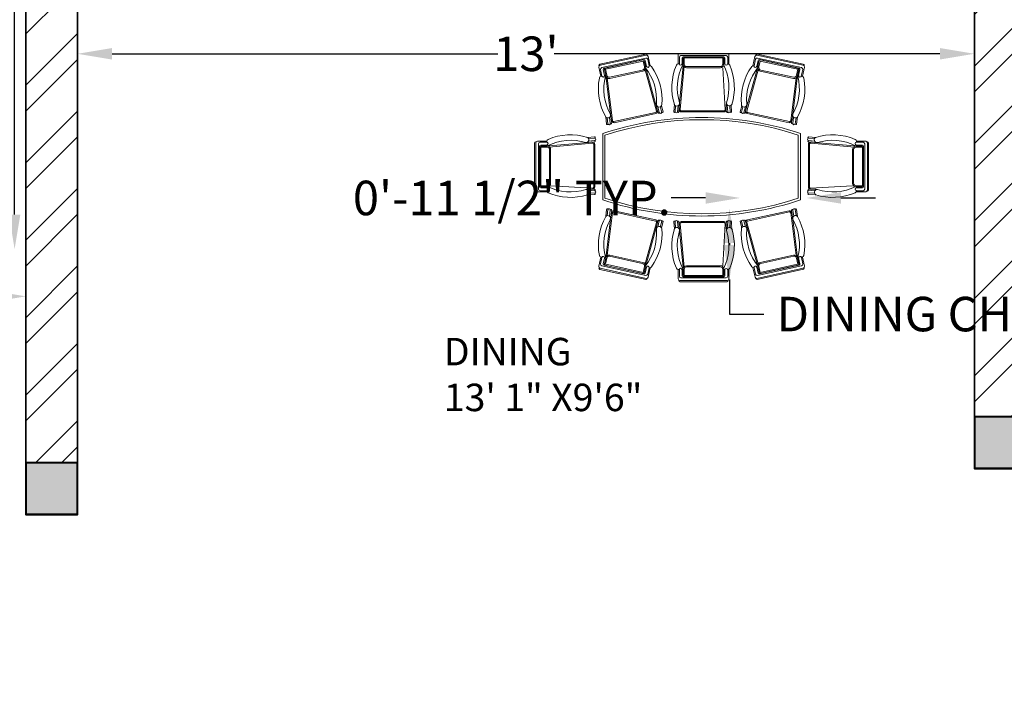
# Model space of a CAD drawing. Units: inches. Extents: x 3614 to 4242, y 2406 to 3033.
# Tile 7 of 10: x 3808 to 3980, y 2749 to 2864. Entities that reach past the tile are written whole.
import ezdxf

# ---------------------------------------------------------------- set-up
doc = ezdxf.new("R2010")
doc.units = ezdxf.units.IN
for name, color, linetype, lineweight in [('A-ANNO-DIMS', 2, 'Continuous', 18), ('A-AREA-IDEN', 7, 'Continuous', 25), ('A-COLS', 7, 'Continuous', 40), ('A-COLS-PATT', 252, 'Continuous', 18), ('A-FURN', 8, 'Continuous', 18), ('A-WALL', 7, 'Continuous', 35), ('A-WALL-PATT', 252, 'Continuous', 13)]:
    doc.layers.add(name, color=color, linetype=linetype, lineweight=lineweight)
doc.styles.get("Standard").update_dxf_attribs({"font": 'arial.ttf'})
doc.dimstyles.get("Standard").update_dxf_attribs({"dimtxt": 6, "dimasz": 6, "dimexe": 0.18, "dimexo": 0.0625, "dimgap": 0.09, "dimtad": 0, "dimtih": 1, "dimtoh": 1, "dimdec": 4, "dimzin": 0, "dimdsep": 46, "dimlunit": 4, "dimtxsty": 'Standard', "dimcen": 0.09, "dimse1": 1, "dimse2": 1, "dimadec": 0, "dimazin": 0, "dimtfac": 1, "dimtdec": 4, "dimtofl": 0, "dimtmove": 0, "dimatfit": 3, "dimfxl": 1, "dimtolj": 1, "dimtzin": 0, "dimarcsym": 0})

# ---------------------------------------------------------------- blocks, each defined once
blk = doc.blocks.new('*D14')
at = {"layer": 'A-ANNO-DIMS', "color": 0, "lineweight": -2, "transparency": 16777216}
for p, q in [((3824.34, 2858.42), (3891.44, 2858.42)), ((3968.34, 2858.42), (3901.24, 2858.42))]:
    blk.add_line(p, q, dxfattribs=at)
at = {"layer": 'A-ANNO-DIMS', "color": 0, "transparency": 16777216}
for points in [[(3824.34, 2859.42), (3824.34, 2857.42), (3818.34, 2858.42)], [(3968.34, 2859.42), (3968.34, 2857.42), (3974.34, 2858.42)]]:
    blk.add_solid(points, dxfattribs=at)
at = {"layer": 'Defpoints', "color": 0, "transparency": 16777216}
for p in [(3974.34, 2858.42), (3818.34, 2819.44), (3974.34, 2819.44)]:
    blk.add_point(p, dxfattribs=at)
at = {"layer": 'A-ANNO-DIMS', "color": 0, "transparency": 16777216, "insert": (3896.34, 2858.42), "char_height": 6, "attachment_point": 5}
blk.add_mtext("\\A1;13'", dxfattribs=at)
blk = doc.blocks.new('*D16')
at = {"layer": 'A-ANNO-DIMS', "color": 0, "lineweight": -2, "transparency": 16777216}
for p, q in [((3703.34, 2816.24), (3745.27, 2816.24)), ((3803.34, 2816.24), (3761.4, 2816.24))]:
    blk.add_line(p, q, dxfattribs=at)
at = {"layer": 'A-ANNO-DIMS', "color": 0, "transparency": 16777216}
for points in [[(3703.34, 2817.24), (3703.34, 2815.24), (3697.34, 2816.24)], [(3803.34, 2817.24), (3803.34, 2815.24), (3809.34, 2816.24)]]:
    blk.add_solid(points, dxfattribs=at)
at = {"layer": 'Defpoints', "color": 0, "transparency": 16777216}
for p in [(3809.34, 2816.24), (3697.34, 2813.05), (3809.34, 2813.05)]:
    blk.add_point(p, dxfattribs=at)
at = {"layer": 'A-ANNO-DIMS', "color": 0, "transparency": 16777216, "insert": (3753.34, 2816.24), "char_height": 6, "attachment_point": 5}
blk.add_mtext('\\A1;9\'-4"', dxfattribs=at)
blk = doc.blocks.new('COLUMN-9X9')
blk.add_lwpolyline([(9, 9), (0, 9), (0, 0), (9, 0)], close=True)
blk = doc.blocks.new('CHAIR-DINING')
for p, q in [((8.3, 12.29), (0.27, 10.54)), ((8.34, 12.11), (0.31, 10.36)), ((8.25, 11.6), (0.6, 9.93)), ((7.92, 11.33), (1.01, 9.82)), ((2.05, 10.02), (7.75, 11.27)), ((2.09, 9.83), (7.79, 11.08)), ((8.01, 10.07), (7.79, 11.08)), ((8.2, 10.12), (7.98, 11.12)), ((8.37, 10.16), (8.15, 11.19)), ((8.84, 10.26), (8.59, 11.38)), ((9.03, 10.26), (8.68, 11.89)), ((0.09, 10.01), (0.44, 8.43)), ((0.38, 9.59), (0.62, 8.47)), ((0.87, 9.6), (1.09, 8.57)), ((1.28, 8.57), (1.05, 9.61)), ((1.08, 8.6), (1.08, 8.6)), ((1.2, 9.84), (2.05, 10.02)), ((1.24, 9.65), (2.09, 9.83)), ((1.47, 8.61), (1.24, 9.65)), ((1.28, 8.55), (1.28, 8.57)), ((2.12, 1.84), (1.28, 8.57)), ((1.47, 8.61), (1.47, 8.58)), ((7.65, 9.5), (1.93, 8.25)), ((7.76, 9.33), (1.98, 8.07)), ((10.11, 2.37), (8.12, 9.58)), ((8.37, 10.15), (8.21, 10.12)), ((8.36, 9.41), (8.22, 9.89)), ((10.3, 2.43), (8.35, 9.46)), ((0.62, 8.47), (0.47, 8.44)), ((2.46, 0.71), (1.53, 8.15)), ((2.27, 0.69), (2.12, 1.84)), ((9.97, 2.14), (2.69, 0.55)), ((10.01, 1.95), (2.73, 0.36)), ((10.39, 2.07), (10.3, 2.4)), ((10.61, 2.12), (10.33, 3.14)), ((11.02, 2.2), (10.77, 3.12)), ((11.27, 2.24), (10.98, 3.3)), ((11.28, 2.23), (11.28, 2.23)), ((1.44, 0.11), (1.29, 1.36)), ((1.67, 0.16), (1.54, 1.21)), ((1.65, 0.13), (1.65, 0.13)), ((2.08, 0.25), (1.95, 1.29)), ((2.32, 0.31), (2.24, 0.93))]:
    blk.add_line(p, q)
for centre, radius, start, end in [((8.33, 12.1), 0.197, 12.3034, 102.3033), ((8.4, 11.83), 0.287, 12.3033, 102.303), ((0.37, 10.08), 0.287, 102.303, 192.3026), ((0.31, 10.35), 0.197, 102.3033, 212.9157), ((7.79, 11.08), 0.191, 12.3033, 102.3033), ((7.96, 11.14), 0.191, 12.3033, 102.303), ((8.31, 11.32), 0.287, 12.3033, 102.303), ((0.66, 9.65), 0.287, 102.303, 192.3026), ((0.84, 8.52), 0.242, 192.3034, 12.3032), ((1.05, 9.64), 0.191, 102.303, 192.3026), ((1.24, 9.65), 0.191, 102.3033, 192.3033), ((1.11, 8.42), 0.153, 71.7142, 102.3033), ((1.13, 8.47), 0.0956, 345.8699, 71.7142), ((1.85, 8.63), 0.382, 187.1284, 282.3033), ((7.55, 9.97), 0.478, 282.3033, 12.3033), ((7.64, 9.89), 0.573, 282.3033, 1.4878), ((8.23, 10.03), 0.0956, 102.3033, 218.7668), ((1.17, 4.36), 8.96, 354.9923, 38.7668), ((8.6, 10.22), 0.241, 194.1944, 8.7091), ((8.94, 9.89), 0.382, 35.4828, 104.8136), ((1.17, 4.36), 9.91, 354.9923, 35.4828), ((9.91, 6.26), 9.91, 169.1238, 209.6143), ((0.55, 8.06), 0.382, 102.3033, 169.1238), ((9.91, 6.26), 8.96, 165.8699, 209.6143), ((1.85, 8.63), 0.573, 187.1284, 282.3033), ((10.57, 3.55, -5.2), 0.477, 176.9365, 356.9364), ((1.66, 1.67), 0.477, 222.431, 27.6701), ((9.93, 2.32), 0.191, 282.3033, 15.4638), ((9.93, 2.32), 0.382, 282.3033, 15.4638), ((10.5, 2.1), 0.11, 193.7607, 13.7605), ((10.81, 2.17), 0.21, 192.3034, 12.3032), ((11.14, 2.23), 0.128, 193.5526, 13.5524), ((1.56, 0.14), 0.118, 192.3034, 12.3032), ((1.87, 0.21), 0.208, 192.3034, 12.3032), ((2.2, 0.28), 0.122, 193.4857, 13.4856), ((2.65, 0.74), 0.382, 187.1284, 282.3033), ((2.65, 0.74), 0.191, 187.1284, 282.3033)]:
    blk.add_arc(centre, radius, start, end)
blk = doc.blocks.new('*D45')
at = {"layer": 'A-ANNO-DIMS', "color": 0, "lineweight": -2, "transparency": 16777216}
for p, q in [((3931.73, 2825.5), (3931.73, 2825.16)), ((3931.73, 2819.16), (3931.73, 2813.16)), ((3931.73, 2813.16), (3937.73, 2813.16))]:
    blk.add_line(p, q, dxfattribs=at)
at = {"layer": 'A-ANNO-DIMS', "color": 0, "transparency": 16777216}
for points in [[(3932.73, 2825.5), (3930.73, 2825.5), (3931.73, 2831.5)], [(3932.73, 2825.16), (3930.73, 2825.16), (3931.73, 2819.16)]]:
    blk.add_solid(points, dxfattribs=at)
at = {"layer": 'Defpoints', "color": 0, "transparency": 16777216}
for p in [(3933.58, 2831.5), (3931.73, 2819.16), (3933.58, 2819.16)]:
    blk.add_point(p, dxfattribs=at)
at = {"layer": 'A-ANNO-DIMS', "color": 0, "transparency": 16777216, "insert": (3992.99, 2813.16), "char_height": 6, "attachment_point": 5}
blk.add_mtext('\\A1;DINING CHAIR 1\'-0 1/2" TYP.', dxfattribs=at)
blk = doc.blocks.new('*D46')
at = {"layer": 'A-ANNO-DIMS', "color": 0, "lineweight": -2, "transparency": 16777216}
for p, q in [((3927.58, 2833.35), (3921.58, 2833.35)), ((3951.13, 2833.36), (3957.13, 2833.36))]:
    blk.add_line(p, q, dxfattribs=at)
at = {"layer": 'A-ANNO-DIMS', "color": 0, "transparency": 16777216}
for points in [[(3927.58, 2834.35), (3927.58, 2832.35), (3933.58, 2833.35)], [(3951.13, 2834.36), (3951.13, 2832.36), (3945.13, 2833.35)]]:
    blk.add_solid(points, dxfattribs=at)
at = {"layer": 'Defpoints', "color": 0, "transparency": 16777216}
for p in [(3933.58, 2833.35), (3933.58, 2831.5), (3945.13, 2831.5)]:
    blk.add_point(p, dxfattribs=at)
at = {"layer": 'A-ANNO-DIMS', "color": 0, "transparency": 16777216, "insert": (3893.88, 2833.35), "char_height": 6, "attachment_point": 5}
blk.add_mtext('\\A1;0\'-11 1/2" TYP.', dxfattribs=at)
blk = doc.blocks.new('*D63')
at = {"layer": 'A-ANNO-DIMS', "color": 0, "lineweight": -2, "transparency": 16777216}
for p, q in [((3807.39, 2928.9), (3807.39, 2882.88)), ((3807.39, 2830.46), (3807.39, 2876.49))]:
    blk.add_line(p, q, dxfattribs=at)
at = {"layer": 'A-ANNO-DIMS', "color": 0, "transparency": 16777216}
for points in [[(3806.39, 2928.9), (3808.39, 2928.9), (3807.39, 2934.9)], [(3806.39, 2830.46), (3808.39, 2830.46), (3807.39, 2824.46)]]:
    blk.add_solid(points, dxfattribs=at)
at = {"layer": 'Defpoints', "color": 0, "transparency": 16777216}
for p in [(3790.82, 2934.9), (3807.39, 2934.9), (3790.82, 2824.46)]:
    blk.add_point(p, dxfattribs=at)
at = {"layer": 'A-ANNO-DIMS', "color": 0, "transparency": 16777216, "insert": (3807.39, 2879.68), "char_height": 6, "attachment_point": 5}
blk.add_mtext('\\A1;KITCHEN COUNTER 9\'-2 1/2"', dxfattribs=at)

msp = doc.modelspace()

# ---------------------------------------------------------------- hatches: boundary and pattern name
at = {"layer": 'A-COLS-PATT'}
h = msp.add_hatch(color=256, dxfattribs=at)
h.dxf.hatch_style = 1
h.paths.add_polyline_path([(3697.336, 2954.34049), (3688.336, 2954.34049), (3688.336, 2945.34049), (3697.336, 2945.34049)])
h.paths.add_polyline_path([(3818.336, 2954.34049), (3809.336, 2954.34049), (3809.336, 2945.34049), (3818.336, 2945.34049)])
h.paths.add_polyline_path([(3818.336, 2787.28572), (3809.336, 2787.28572), (3809.336, 2778.34049), (3818.336, 2778.34049)])
h.paths.add_polyline_path([(3697.336, 2742.34049), (3688.336, 2742.34049), (3688.336, 2733.34049), (3697.336, 2733.34049)])
h.paths.add_polyline_path([(3697.336, 2583.37355), (3688.336, 2583.37355), (3688.336, 2574.37355), (3697.336, 2574.37355)])
h.paths.add_polyline_path([(3899.336, 2583.34049), (3890.336, 2583.34049), (3890.336, 2574.34049), (3899.336, 2574.34049)])
h.paths.add_polyline_path([(3983.336, 2583.34049), (3974.336, 2583.34049), (3974.336, 2574.34049), (3983.336, 2574.34049)])
h.paths.add_polyline_path([(4153.336, 2583.34049), (4144.336, 2583.34049), (4144.336, 2574.34049), (4153.336, 2574.34049)])
h.paths.add_polyline_path([(4153.336, 2742.34049), (4144.336, 2742.34049), (4144.336, 2733.34049), (4153.336, 2733.34049)])
h.paths.add_polyline_path([(4153.336, 2795.34049), (4144.336, 2795.34049), (4144.336, 2786.34049), (4153.336, 2786.34049)])
h.paths.add_polyline_path([(3983.336, 2795.31105), (3974.336, 2795.31105), (3974.336, 2786.34049), (3983.336, 2786.34049)])
h.paths.add_polyline_path([(4153.336, 2954.34049), (4144.36882, 2954.34049), (4144.36882, 2945.34049), (4153.336, 2945.34049)])
h.paths.add_polyline_path([(3982.96188, 2954.34049), (3973.96188, 2954.34049), (3973.96188, 2945.34049), (3982.96188, 2945.34049)])
at = {"layer": 'A-WALL-PATT'}
h = msp.add_hatch(dxfattribs=at)
h.set_pattern_fill('ANSI32', color=256)
h.paths.add_polyline_path([(4041.01458, 2954.34049), (3982.96188, 2954.34049), (3982.96188, 2945.34049), (3983.336, 2945.34049), (4041.01458, 2945.34049)])
h.paths.add_polyline_path([(3973.96188, 2954.34049), (3960.11861, 2954.34049), (3960.11861, 2945.34049), (3973.96188, 2945.34049)])
h.paths.add_polyline_path([(3936.11861, 2954.34049), (3901.17016, 2954.34049), (3901.17016, 2945.34049), (3913.336, 2945.34049), (3913.336, 2896.34049, -0.050382044), (3919.336, 2895.73437), (3919.336, 2945.34049), (3936.11861, 2945.34049)])
h.paths.add_polyline_path([(3983.336, 2945.34049), (3982.96188, 2945.34049), (3974.336, 2945.34049), (3974.336, 2873.34049), (3974.336, 2795.31105), (3983.336, 2795.31105), (3983.336, 2867.34049)])
h.paths.add_polyline_path([(3974.336, 2872.34049), (3919.336, 2872.34049), (3858.336, 2872.34049), (3858.336, 2866.34049), (3919.336, 2866.34049), (3974.336, 2866.34049)])
h.paths.add_polyline_path([(3877.17016, 2954.34049), (3852.34021, 2954.34049), (3852.34021, 2945.34049), (3852.336, 2896.34049), (3858.336, 2896.34049), (3858.336, 2945.34049), (3877.17016, 2945.34049)])
h.paths.add_polyline_path([(3871.94212, 2902.34049), (3858.336, 2902.34049), (3858.336, 2896.34049), (3871.336, 2896.34049, -0.050382044)], flags=0)
h.paths.add_polyline_path([(3913.336, 2902.34049), (3901.336, 2902.34049), (3901.336, 2896.34049), (3913.336, 2896.34049)], flags=17)
h.paths.add_polyline_path([(3858.336, 2872.34049), (3852.336, 2872.34049), (3852.336, 2866.34049), (3858.336, 2866.34049)])
h.paths.add_polyline_path([(3809.336, 2954.34049), (3764.4617, 2954.34049), (3764.4617, 2945.34049), (3809.336, 2945.34049)])
h.paths.add_polyline_path([(3716.4617, 2954.34049), (3697.336, 2954.34049), (3697.336, 2945.34049), (3716.4617, 2945.34049)])
h.paths.add_polyline_path([(3697.336, 2945.34049), (3688.336, 2945.34049), (3688.336, 2894.73438), (3697.336, 2894.73438)])
h = msp.add_hatch(dxfattribs=at)
h.set_pattern_fill('ANSI32', color=256)
h.paths.add_polyline_path([(4153.336, 2945.34049), (4144.336, 2945.34049), (4144.336, 2902.95478), (4153.336, 2902.95478)])
h.paths.add_polyline_path([(4144.36882, 2954.34049), (4089.01458, 2954.34049), (4089.01458, 2945.34049), (4144.36882, 2945.34049)])
h.paths.add_polyline_path([(3818.336, 2945.34049), (3809.336, 2945.34049), (3809.336, 2787.28572), (3818.336, 2787.28572)])
h.paths.add_polyline_path([(3697.336, 2846.73438), (3688.336, 2846.73438), (3688.336, 2742.34049), (3697.336, 2742.34049)])
h.paths.add_polyline_path([(3854.336, 2742.34049), (3853.36389, 2742.34049), (3818.336, 2742.34049), (3809.336, 2742.34049), (3697.336, 2742.34049), (3697.336, 2733.34049), (3809.336, 2733.34049), (3854.336, 2733.34049)])
h.paths.add_polyline_path([(3697.336, 2733.34049), (3688.336, 2733.34049), (3688.336, 2690.05693), (3697.336, 2690.05693)])
h.paths.add_polyline_path([(3697.336, 2642.05693), (3688.336, 2642.05693), (3688.336, 2583.37355), (3697.336, 2583.37355)])
h.paths.add_polyline_path([(3726.39802, 2583.34049), (3697.336, 2583.34049), (3697.336, 2574.34049), (3726.39802, 2574.34049)])
h.paths.add_polyline_path([(3842.336, 2583.34049), (3818.336, 2583.34049), (3809.336, 2583.34049), (3774.39802, 2583.34049), (3774.39802, 2574.34049), (3809.336, 2574.34049), (3842.336, 2574.34049)])
h.paths.add_polyline_path([(3890.336, 2583.34049), (3878.336, 2583.34049), (3878.336, 2574.34049), (3890.336, 2574.34049)])
h = msp.add_hatch(dxfattribs=at)
h.set_pattern_fill('ANSI32', color=256)
h.paths.add_polyline_path([(3899.336, 2733.34049), (3899.336, 2742.34049), (3890.336, 2742.34049), (3890.336, 2583.34049), (3899.336, 2583.34049)])
h.paths.add_polyline_path([(3983.336, 2733.34049), (3995.336, 2733.34049), (3995.336, 2742.34049), (3983.336, 2742.34049), (3974.336, 2742.34049), (3974.336, 2583.34049), (3983.336, 2583.34049)])
h.paths.add_polyline_path([(3974.336, 2583.34049), (3899.336, 2583.34049), (3899.336, 2574.34049), (3974.336, 2574.34049)])
h.paths.add_polyline_path([(4045.73114, 2583.34049), (3983.336, 2583.34049), (3983.336, 2574.34049), (4045.73114, 2574.34049)])
h.paths.add_polyline_path([(4144.336, 2583.34049), (4093.73114, 2583.34049), (4093.73114, 2574.34049), (4144.336, 2574.34049)])
h.paths.add_polyline_path([(4153.336, 2639.00845), (4144.336, 2639.00845), (4144.336, 2583.34049), (4153.336, 2583.34049)])
h.paths.add_polyline_path([(4153.336, 2733.34049), (4144.336, 2733.34049), (4144.336, 2687.00845), (4153.336, 2687.00845)])
h.paths.add_polyline_path([(4144.336, 2742.34049), (4096.76112, 2742.34049, -0.076320834), (4098.14294, 2733.34049), (4144.336, 2733.34049)])
h.paths.add_polyline_path([(4068.14294, 2742.34049), (4056.14294, 2742.34049), (4031.336, 2742.34049, -0.063254224), (4030.19285, 2733.34049), (4068.14294, 2733.34049)])
h.paths.add_polyline_path([(4144.336, 2795.34049), (4042.336, 2795.34049), (4042.336, 2786.34049), (4144.336, 2786.34049)])
h.paths.add_polyline_path([(4153.336, 2854.95478), (4144.336, 2854.95478), (4144.336, 2795.34049), (4153.336, 2795.34049)])

# ---------------------------------------------------------------- linework, layer by layer
at = {"layer": 'A-FURN'}
for p, q in [((3922.82983, 2858.29837), (3922.82981, 2856.67394)), ((3923.02093, 2857.8206), (3923.02092, 2856.67394)), ((3931.14309, 2858.10721), (3923.3076, 2858.10726)), ((3923.49871, 2857.72504), (3923.49869, 2856.67393)), ((3923.68233, 2856.63157), (3923.68233, 2857.69683)), ((3930.76087, 2857.9161), (3923.68982, 2857.91615)), ((3923.87343, 2857.88793), (3930.58343, 2857.88793)), ((3923.87343, 2856.63157), (3923.87343, 2857.69683)), ((3923.87343, 2857.69683), (3930.58343, 2857.69683)), ((3930.58343, 2856.66104), (3930.58343, 2857.69683)), ((3930.77454, 2856.67065), (3930.77454, 2857.69683)), ((3930.95198, 2856.67389), (3930.95198, 2857.72499)), ((3931.42975, 2856.67389), (3931.42975, 2857.82054)), ((3931.62086, 2856.63232), (3931.62086, 2858.29832)), ((3923.01445, 2856.67441), (3922.86495, 2856.67441)), ((3923.07454, 2849.87451), (3923.65867, 2856.32445)), ((3923.16044, 2848.70423), (3923.85057, 2856.32445)), ((3923.49867, 2856.70429), (3923.49873, 2856.70491)), ((3923.68519, 2856.6172), (3923.68642, 2856.63078)), ((3930.10566, 2856.18327), (3924.25618, 2856.18327)), ((3930.17748, 2855.99216), (3924.25618, 2855.99216)), ((3930.99473, 2848.69753), (3930.59251, 2855.98182)), ((3930.9483, 2856.67065), (3930.78946, 2856.67065)), ((3930.94127, 2856.64313), (3930.93959, 2856.67171)), ((3931.43017, 2856.6484), (3931.429, 2856.67171)), ((3922.03956, 2848.33797), (3922.15359, 2849.59779)), ((3922.24897, 2848.30477), (3922.24904, 2848.30589)), ((3922.27521, 2848.33797), (3922.36724, 2849.38276)), ((3922.69211, 2848.33797), (3922.79272, 2849.38159)), ((3922.93698, 2848.34511), (3922.99185, 2848.96492)), ((3922.97011, 2848.72146), (3923.07454, 2849.87451)), ((3930.80391, 2848.49588), (3923.35077, 2848.49588)), ((3930.80391, 2848.30477), (3923.35077, 2848.30477)), ((3931.18555, 2848.70806), (3931.13769, 2849.57484)), ((3931.2038, 2848.34033), (3931.18226, 2848.68338)), ((3931.429, 2848.33797), (3931.35985, 2849.51543)), ((3931.84591, 2848.33797), (3931.79587, 2849.33815)), ((3932.09871, 2848.32111), (3932.03174, 2849.44774)), ((3932.09968, 2848.30477), (3932.09961, 2848.30589)), ((3898.32537, 2843.21638), (3899.9498, 2843.2164)), ((3899.94933, 2843.03177), (3899.94933, 2843.18126)), ((3908.28577, 2844.00665), (3907.02595, 2843.89262)), ((3908.28577, 2843.77101), (3907.24099, 2843.67897)), ((3908.28577, 2843.3541), (3907.24215, 2843.25349)), ((3908.31897, 2843.79724), (3908.31786, 2843.79717)), ((3909.69472, 2844.54018), (3909.69472, 2833.01769)), ((3910.07694, 2844.2642), (3910.07694, 2833.29345)), ((3943.71216, 2844.29393), (3943.71216, 2833.29033)), ((3944.09438, 2844.57043), (3944.09438, 2833.01451)), ((3945.46538, 2843.79724), (3945.4665, 2843.79717)), ((3945.49859, 2844.00665), (3946.7584, 2843.89262)), ((3945.49859, 2843.77101), (3946.54337, 2843.67897)), ((3945.49859, 2843.3541), (3946.54221, 2843.25349)), ((3955.45898, 2843.21638), (3953.83455, 2843.2164)), ((3953.83502, 2843.03177), (3953.83502, 2843.18126)), ((3897.84765, 2834.71201), (3897.8476, 2842.92972)), ((3898.03876, 2834.71202), (3898.03871, 2842.92972)), ((3898.51654, 2834.90312), (3898.51649, 2842.73861)), ((3898.70764, 2835.28534), (3898.7076, 2842.3564)), ((3898.73581, 2842.17278), (3898.73581, 2835.46278)), ((3898.80315, 2843.02528), (3899.9498, 2843.02529)), ((3898.8987, 2842.54751), (3899.94981, 2842.54752)), ((3899.99218, 2842.36389), (3898.92692, 2842.36389)), ((3898.92692, 2842.17278), (3898.92692, 2835.46278)), ((3899.99218, 2842.17278), (3898.92692, 2842.17278)), ((3899.91945, 2842.54754), (3899.91883, 2842.54748)), ((3900.00655, 2842.36103), (3899.99296, 2842.3598)), ((3907.90228, 2843.0761), (3900.29929, 2842.38754)), ((3907.91952, 2842.88577), (3900.29929, 2842.19565)), ((3900.44048, 2835.94056), (3900.44048, 2841.79004)), ((3900.63158, 2835.86873), (3900.63158, 2841.79004)), ((3908.27863, 2843.10923), (3907.65883, 2843.05436)), ((3908.12786, 2835.2423), (3908.12786, 2842.69544)), ((3908.31897, 2835.2423), (3908.31897, 2842.69544)), ((3945.46538, 2835.2423), (3945.46538, 2842.69544)), ((3945.50572, 2843.10923), (3946.12553, 2843.05436)), ((3945.65649, 2835.2423), (3945.65649, 2842.69544)), ((3945.86484, 2842.88577), (3953.48507, 2842.19565)), ((3945.88208, 2843.0761), (3953.48507, 2842.38754)), ((3953.15277, 2835.86873), (3953.15277, 2841.79004)), ((3953.34388, 2835.94056), (3953.34388, 2841.79004)), ((3953.77781, 2842.36103), (3953.79139, 2842.3598)), ((3953.79218, 2842.36389), (3954.85744, 2842.36389)), ((3953.79218, 2842.17278), (3954.85744, 2842.17278)), ((3954.98121, 2843.02528), (3953.83455, 2843.02529)), ((3954.88565, 2842.54751), (3953.83455, 2842.54752)), ((3953.86491, 2842.54754), (3953.86553, 2842.54748)), ((3954.85744, 2842.17278), (3954.85744, 2835.46278)), ((3955.04855, 2842.17278), (3955.04855, 2835.46278)), ((3955.07671, 2835.28534), (3955.07676, 2842.3564)), ((3955.26782, 2834.90312), (3955.26787, 2842.73861)), ((3955.74559, 2834.71202), (3955.74564, 2842.92972)), ((3955.9367, 2834.71201), (3955.93675, 2842.92972)), ((3899.94986, 2834.61646), (3898.8032, 2834.61646)), ((3899.94986, 2835.09424), (3898.89875, 2835.09424)), ((3899.9627, 2835.46278), (3898.92692, 2835.46278)), ((3899.95309, 2835.27168), (3898.92692, 2835.27168)), ((3899.98062, 2835.10494), (3899.95203, 2835.10662)), ((3899.97534, 2834.61605), (3899.95203, 2834.61721)), ((3899.95309, 2835.09791), (3899.95309, 2835.25676)), ((3907.92622, 2835.05148), (3900.64192, 2835.4537)), ((3907.91568, 2834.86066), (3907.0489, 2834.90852)), ((3908.28577, 2834.61721), (3907.10832, 2834.68636)), ((3908.28341, 2834.84241), (3907.94036, 2834.86396)), ((3945.49859, 2834.61721), (3946.67604, 2834.68636)), ((3945.50095, 2834.84241), (3945.84399, 2834.86396)), ((3945.85814, 2835.05148), (3953.14243, 2835.4537)), ((3945.86868, 2834.86066), (3946.73546, 2834.90852)), ((3953.80374, 2835.10494), (3953.83233, 2835.10662)), ((3953.80902, 2834.61605), (3953.83233, 2834.61721)), ((3953.82165, 2835.46278), (3954.85744, 2835.46278)), ((3953.83127, 2835.27168), (3954.85744, 2835.27168)), ((3953.83127, 2835.09791), (3953.83127, 2835.25676)), ((3953.8345, 2835.09424), (3954.8856, 2835.09424)), ((3953.8345, 2834.61646), (3954.98116, 2834.61646)), ((3899.99142, 2834.42535), (3898.32543, 2834.42535)), ((3908.30263, 2833.94751), (3907.17601, 2834.01447)), ((3908.28577, 2834.20031), (3907.28559, 2834.25034)), ((3908.31897, 2833.94654), (3908.31786, 2833.9466)), ((3945.46538, 2833.94654), (3945.4665, 2833.9466)), ((3945.48172, 2833.94751), (3946.60835, 2834.01447)), ((3945.49859, 2834.20031), (3946.49877, 2834.25034)), ((3953.79293, 2834.42535), (3955.45893, 2834.42535)), ((3922.03956, 2829.21982), (3922.15359, 2827.96001)), ((3922.24897, 2829.25302), (3922.24904, 2829.25191)), ((3922.27521, 2829.21982), (3922.36724, 2828.17504)), ((3922.69211, 2829.21982), (3922.79272, 2828.1762)), ((3922.93698, 2829.21269), (3922.99185, 2828.59288)), ((3922.97011, 2828.83633), (3923.07454, 2827.68329)), ((3923.16044, 2828.85357), (3923.85057, 2821.23334)), ((3930.80391, 2829.25302), (3923.35077, 2829.25302)), ((3930.80391, 2829.06192), (3923.35077, 2829.06192)), ((3930.99473, 2828.86027), (3930.59251, 2821.57598)), ((3931.18555, 2828.84973), (3931.13769, 2827.98295)), ((3931.2038, 2829.21746), (3931.18226, 2828.87442)), ((3931.429, 2829.21982), (3931.35985, 2828.04237)), ((3931.84591, 2829.21982), (3931.79587, 2828.21964)), ((3932.09871, 2829.23668), (3932.03174, 2828.11006)), ((3932.09968, 2829.25302), (3932.09961, 2829.25191)), ((3923.07454, 2827.68329), (3923.65867, 2821.23334)), ((3922.82983, 2819.25942), (3922.82981, 2820.88386)), ((3923.01445, 2820.88339), (3922.86495, 2820.88339)), ((3923.02093, 2819.7372), (3923.02092, 2820.88386)), ((3923.49867, 2820.8535), (3923.49873, 2820.85288)), ((3923.49871, 2819.83276), (3923.49869, 2820.88386)), ((3923.68233, 2820.92623), (3923.68233, 2819.86097)), ((3923.68519, 2820.9406), (3923.68642, 2820.92702)), ((3923.87343, 2820.92623), (3923.87343, 2819.86097)), ((3930.17748, 2821.56564), (3924.25618, 2821.56564)), ((3930.10566, 2821.37453), (3924.25618, 2821.37453)), ((3930.58343, 2820.89676), (3930.58343, 2819.86097)), ((3930.77454, 2820.88714), (3930.77454, 2819.86097)), ((3930.9483, 2820.88714), (3930.78946, 2820.88714)), ((3930.94127, 2820.91467), (3930.93959, 2820.88608)), ((3930.95198, 2820.88391), (3930.95198, 2819.8328)), ((3931.43017, 2820.90939), (3931.429, 2820.88608)), ((3931.42975, 2820.88391), (3931.42975, 2819.73725)), ((3931.62086, 2820.92548), (3931.62086, 2819.25948)), ((3931.14309, 2819.45059), (3923.3076, 2819.45054)), ((3930.76087, 2819.6417), (3923.68982, 2819.64165)), ((3923.87343, 2819.86097), (3930.58343, 2819.86097)), ((3923.87343, 2819.66986), (3930.58343, 2819.66986)), ((3931.3342, 2818.97282), (3923.1165, 2818.97276)), ((3931.3342, 2818.78171), (3923.1165, 2818.78166))]:
    msp.add_line(p, q, dxfattribs=at)
for centre, radius, start, end in [((3923.3076, 2857.82059), 0.28666, 89.9996381, 179.999275), ((3923.68982, 2857.72504), 0.19111, 89.9996381, 179.999275), ((3923.87343, 2857.69683), 0.19111, 90, 180), ((3930.58343, 2857.69683), 0.19111, 0, 90), ((3930.76087, 2857.72499), 0.19111, 0, 89.9996381), ((3931.14309, 2857.82054), 0.28666, 0, 89.9996381), ((3931.6278, 2852.54013), 9.91456, 156.8204824, 197.3110234), ((3922.86495, 2856.29219), 0.38222, 90, 156.8204824), ((3931.6278, 2852.54013), 8.95902, 153.5665946, 197.3110234), ((3923.24766, 2856.68072), 0.24162, 180.000076, 359.999924), ((3923.49057, 2856.52128), 0.15313, 59.410873, 90), ((3923.51987, 2856.57084), 0.09555, 333.5665946, 59.410873), ((3924.25618, 2856.56549), 0.57333, 174.8251214, 270), ((3931.6278, 2852.54013), 8.95902, 152.2307223, 152.4302915), ((3924.25618, 2856.56549), 0.38222, 174.8251214, 270), ((3930.10566, 2856.66104), 0.47777, 270, 0), ((3930.17748, 2856.56549), 0.57333, 270, 351.0504472), ((3930.78946, 2856.5751), 0.09555, 90, 206.4634741), ((3922.68363, 2852.54013), 8.95902, 342.6889766, 26.4634741), ((3931.1819, 2856.68072), 0.23333, 180.000076, 359.999924), ((3931.44649, 2856.29219), 0.38222, 23.1795176, 90), ((3922.68363, 2852.54013), 9.91456, 342.6889766, 23.1795176), ((3922.15697, 2848.33728), 0.1178, 180.000076, 359.999924), ((3922.58115, 2849.80894), 0.47686, 195.3669467, 15.3667947), ((3922.48298, 2848.33728), 0.20821, 180.000076, 359.999924), ((3922.81275, 2848.33979), 0.12159, 181.1824337, 1.1822816), ((3923.35077, 2848.68699), 0.38222, 174.8251214, 270), ((3923.35077, 2848.68699), 0.19111, 174.8251214, 270), ((3930.80391, 2848.68699), 0.38222, 270, 3.1605363), ((3930.80391, 2848.68699), 0.19111, 270, 3.1605363), ((3931.31411, 2848.34232), 0.10978, 181.4573887, 1.4572366), ((3931.7224, 2849.82282), 0.48828, 173.9478508, 343.3079431), ((3931.6342, 2848.34511), 0.21034, 180.000076, 359.999924), ((3931.96801, 2848.33673), 0.12807, 181.2492726, 1.2491205), ((3926.93992, 2792.95024), 54.39594, 71.6172783, 108.4834683), ((3926.93992, 2792.95024), 54.01373, 71.9095396, 108.1917482), ((3898.03969, 2842.93357), 0.1967, 90.0021394, 180), ((3898.32538, 2842.92972), 0.28666, 90.0007254, 180.0003625), ((3900.33155, 2843.18126), 0.38222, 113.1795173, 180), ((3904.08361, 2834.41841), 8.95902, 72.688977, 116.4334046), ((3904.08361, 2834.41841), 9.91456, 72.688977, 113.1795173), ((3906.8148, 2843.46507), 0.47686, 254.6332057, 74.6330535), ((3908.28395, 2843.23346), 0.12159, 268.8177181, 88.8175663), ((3908.28646, 2843.88924), 0.1178, 270.0000767, 89.9999233), ((3908.28646, 2843.56323), 0.20821, 270.0000767, 89.9999233), ((3945.4979, 2843.56323), 0.20821, 90.0000767, 269.9999233), ((3945.50041, 2843.23346), 0.12159, 91.1824337, 271.1822819), ((3945.4979, 2843.88924), 0.1178, 90.0000767, 269.9999233), ((3946.96955, 2843.46507), 0.47686, 105.3669465, 285.3667943), ((3949.70075, 2834.41841), 9.91456, 66.8204827, 107.311023), ((3949.70075, 2834.41841), 8.95902, 63.5665954, 107.311023), ((3953.45281, 2843.18126), 0.38222, 0, 66.8204827), ((3955.45898, 2842.92972), 0.28666, 359.9996375, 89.9992746), ((3955.74467, 2842.93357), 0.1967, 0, 89.9978605), ((3898.80315, 2842.73861), 0.28666, 90.0007254, 180.0003625), ((3898.89871, 2842.3564), 0.19111, 90.0007254, 180.0003625), ((3898.92692, 2842.17278), 0.19111, 90, 180), ((3904.08361, 2834.41841), 8.95902, 117.5697085, 117.7692773), ((3899.94303, 2842.79855), 0.24162, 270.0000767, 89.9999233), ((3900.10247, 2842.55565), 0.15313, 180, 210.5891277), ((3900.0529, 2842.52635), 0.09555, 210.5891277, 296.4334046), ((3900.05826, 2841.79004), 0.57333, 0, 95.174878), ((3900.05826, 2841.79004), 0.38222, 0, 95.174878), ((3907.93675, 2842.69544), 0.38222, 0, 95.174878), ((3907.93675, 2842.69544), 0.19111, 0, 95.174878), ((3945.8476, 2842.69544), 0.38222, 84.825122, 180), ((3945.8476, 2842.69544), 0.19111, 84.825122, 180), ((3953.7261, 2841.79004), 0.57333, 84.825122, 180), ((3953.7261, 2841.79004), 0.38222, 84.825122, 180), ((3953.84133, 2842.79855), 0.24162, 90.0000767, 269.9999233), ((3953.73146, 2842.52635), 0.09555, 243.5665954, 329.4108723), ((3953.68189, 2842.55565), 0.15313, 329.4108723, 0), ((3949.70075, 2834.41841), 8.95902, 62.2307227, 62.4302915), ((3954.85744, 2842.17278), 0.19111, 0, 90), ((3954.88565, 2842.3564), 0.19111, 359.9996375, 89.9992746), ((3954.98121, 2842.73861), 0.28666, 359.9996375, 89.9992746), ((3898.03969, 2834.721), 0.1967, 180, 269.9999233), ((3898.32543, 2834.71202), 0.28666, 180.0003625, 270), ((3898.8032, 2834.90313), 0.28666, 180.0003625, 270), ((3898.89875, 2835.28535), 0.19111, 180.0003625, 270), ((3898.92692, 2835.46278), 0.19111, 180, 270), ((3899.94303, 2834.86431), 0.23333, 270.0000767, 89.9999233), ((3900.33155, 2834.59972), 0.38222, 180, 246.8204827), ((3900.04865, 2835.25676), 0.09555, 63.5365262, 180), ((3899.9627, 2835.94056), 0.47777, 270, 0), ((3904.08361, 2843.36258), 8.95902, 243.5365262, 287.311023), ((3900.05826, 2835.86873), 0.57333, 278.9495528, 0), ((3906.80092, 2834.32382), 0.48828, 286.6920574, 96.0521489), ((3907.93675, 2835.2423), 0.38222, 266.8394633, 0), ((3907.93675, 2835.2423), 0.19111, 266.8394633, 0), ((3908.28143, 2834.7321), 0.10978, 268.5427632, 88.5426113), ((3908.27863, 2834.41201), 0.21034, 270.0000767, 89.9999233), ((3945.50572, 2834.41201), 0.21034, 90.0000767, 269.9999233), ((3945.50293, 2834.7321), 0.10978, 91.4573887, 271.4572368), ((3945.8476, 2835.2423), 0.38222, 180, 273.1605367), ((3945.8476, 2835.2423), 0.19111, 180, 273.1605367), ((3946.98343, 2834.32382), 0.48828, 83.9478511, 253.3079426), ((3949.70075, 2843.36258), 8.95902, 252.688977, 296.4634738), ((3953.7261, 2835.86873), 0.57333, 180, 261.0504472), ((3953.82165, 2835.94056), 0.47777, 180, 270), ((3953.45281, 2834.59972), 0.38222, 293.1795173, 0), ((3953.84133, 2834.86431), 0.23333, 90.0000767, 269.9999233), ((3953.73571, 2835.25676), 0.09555, 0, 116.4634738), ((3954.85744, 2835.46278), 0.19111, 270, 0), ((3954.8856, 2835.28535), 0.19111, 270, 359.9996375), ((3954.98116, 2834.90313), 0.28666, 270, 359.9996375), ((3955.45893, 2834.71202), 0.28666, 270, 359.9996375), ((3955.74467, 2834.721), 0.1967, 270.0000767, 0), ((3904.08361, 2843.36258), 9.91456, 246.8204827, 287.311023), ((3908.28701, 2834.07821), 0.12807, 268.7508802, 88.7507268), ((3926.89929, 2884.35721), 54.14558, 251.4733019, 288.5161235), ((3926.89929, 2884.35721), 53.76336, 251.766145, 288.2232229), ((3945.49735, 2834.07821), 0.12807, 91.2492732, 271.2491198), ((3949.70075, 2843.36258), 9.91456, 252.688977, 293.1795173), ((3922.48298, 2829.22051), 0.20821, 0.000076, 179.999924), ((3931.6342, 2829.21269), 0.21034, 0.000076, 179.999924), ((3931.6278, 2825.01766), 9.91456, 162.6889766, 203.1795176), ((3922.15697, 2829.22051), 0.1178, 0.000076, 179.999924), ((3922.58115, 2827.74885), 0.47686, 344.6332053, 164.6330533), ((3922.81275, 2829.218), 0.12159, 358.8177184, 178.8175663), ((3923.35077, 2828.87081), 0.38222, 90, 185.1748786), ((3923.35077, 2828.87081), 0.19111, 90, 185.1748786), ((3930.80391, 2828.87081), 0.38222, 356.8394637, 90), ((3930.80391, 2828.87081), 0.19111, 356.8394637, 90), ((3931.31411, 2829.21548), 0.10978, 358.5427634, 178.5426113), ((3931.7224, 2827.73497), 0.48828, 16.6920569, 186.0521492), ((3922.68363, 2825.01766), 9.91456, 336.8204824, 17.3110234), ((3931.96801, 2829.22106), 0.12807, 358.7508795, 178.7507274), ((3931.6278, 2825.01766), 8.95902, 162.6889766, 206.4334054), ((3922.68363, 2825.01766), 8.95902, 333.5365259, 17.3110234), ((3922.86495, 2821.2656), 0.38222, 203.1795176, 270), ((3923.24766, 2820.87708), 0.24162, 0.000076, 179.999924), ((3923.49057, 2821.03652), 0.15313, 270, 300.589127), ((3923.51987, 2820.98695), 0.09555, 300.589127, 26.4334054), ((3924.25618, 2820.99231), 0.57333, 90, 185.1748786), ((3931.6278, 2825.01766), 8.95902, 207.5697085, 207.7692777), ((3924.25618, 2820.99231), 0.38222, 90, 185.1748786), ((3930.10566, 2820.89676), 0.47777, 0, 90), ((3930.17748, 2820.99231), 0.57333, 8.9495528, 90), ((3930.78946, 2820.9827), 0.09555, 153.5365259, 270), ((3931.1819, 2820.87708), 0.23333, 0.000076, 179.999924), ((3931.44649, 2821.2656), 0.38222, 270, 336.8204824), ((3923.1165, 2819.25943), 0.28666, 180.000725, 270.0003618), ((3923.3076, 2819.7372), 0.28666, 180.000725, 270.0003618), ((3923.68982, 2819.83276), 0.19111, 180.000725, 270.0003618), ((3923.87343, 2819.86097), 0.19111, 180, 270), ((3930.58343, 2819.86097), 0.19111, 270, 0), ((3930.76087, 2819.8328), 0.19111, 270.0003618, 0), ((3931.14309, 2819.73725), 0.28666, 270.0003618, 0), ((3931.3342, 2819.25948), 0.28666, 270.0003618, 0), ((3923.11264, 2818.97374), 0.1967, 180.0021387, 270), ((3931.32521, 2818.97374), 0.1967, 270, 359.999924)]:
    msp.add_arc(centre, radius, start, end, dxfattribs=at)
at = {"layer": 'A-WALL'}
for p, q in [((3809.336, 2945.34049), (3809.336, 2778.34049)), ((3818.336, 2945.34049), (3818.336, 2778.34049)), ((3974.336, 2873.34049), (3974.336, 2786.34049)), ((3974.336, 2786.34049), (3983.336, 2786.34049)), ((3818.336, 2778.34049), (3809.336, 2778.34049))]:
    msp.add_line(p, q, dxfattribs=at)

# ---------------------------------------------------------------- block references
at = {"layer": 'A-COLS'}
for p in [(3974.336, 2786.31056), (3809.336, 2778.28523)]:
    msp.add_blockref('COLUMN-9X9', p, dxfattribs=at)
at = {"layer": 'A-FURN'}
msp.add_blockref('CHAIR-DINING', (3908.929, 2846.079), dxfattribs=at)
at = {"layer": 'A-FURN', "extrusion": (0, 0, -1), "zscale": -1}
msp.add_blockref('CHAIR-DINING', (-3944.85536, 2846.079), dxfattribs=at)
at = {"layer": 'A-FURN', "extrusion": (0, 0, -1), "zscale": -1, "rotation": 180}
msp.add_blockref('CHAIR-DINING', (-3908.929, 2831.47865), dxfattribs=at)
at = {"layer": 'A-FURN', "rotation": 180.0148602316128}
msp.add_blockref('CHAIR-DINING', (3944.85937, 2831.48331), dxfattribs=at)

# ---------------------------------------------------------------- texts
at = {"layer": 'A-AREA-IDEN', "insert": (3882.05253, 2809.02184), "char_height": 4.7777047, "attachment_point": 1}
msp.add_mtext_dynamic_manual_height_columns('DINING\\P13\' 1" X9\'6"', width=66.2541682, gutter_width=12.5, heights=[0], dxfattribs=at)

# ---------------------------------------------------------------- dimensions: what is measured, and where the dimension line sits
at = {"layer": 'A-ANNO-DIMS'}
for base, p1, p2, angle, text, picture, middle in [((3807.38582, 2934.90029), (3790.82041, 2824.46424), (3790.82041, 2934.90029), 90, 'KITCHEN COUNTER <>', '*D63', (3807.38582, 2879.68227)), ((3933.57628, 2833.35064), (3945.12771, 2831.50281), (3933.57676, 2831.49982), 180.0148602, '<> TYP.', '*D46', (3893.87851, 2833.34753)), ((3931.72914, 2819.16048), (3933.57676, 2831.49982), (3933.57996, 2819.16096), 270.0148602, 'DINING CHAIR <> TYP.', '*D45', (3992.98508, 2813.16048))]:
    dim = msp.add_linear_dim(base=base, p1=p1, p2=p2, angle=angle, text=text, dimstyle='Standard', override={"dimdec": 1, "dimlfac": 1, "dimrnd": 0, "dimzin": 1, "dimdsep": 46, "dimlunit": 4, "dimfrac": 2}, dxfattribs=at)
    dim.commit()
    dim.dimension.update_dxf_attribs({"geometry": picture, "text_midpoint": middle})
for base, p1, p2, picture, middle in [((3974.336, 2858.41862), (3818.336, 2819.44433), (3974.336, 2819.44433), '*D14', (3896.336, 2858.41862)), ((3809.336, 2816.23511), (3697.336, 2813.04672), (3809.336, 2813.04672), '*D16', (3753.336, 2816.23511))]:
    dim = msp.add_linear_dim(base=base, p1=p1, p2=p2, dimstyle='Standard', override={"dimclrd": 0, "dimclre": 0, "dimclrt": 0}, dxfattribs=at)
    dim.commit()
    dim.dimension.update_dxf_attribs({"geometry": picture, "text_midpoint": middle})

doc.saveas('drawing.dxf')
